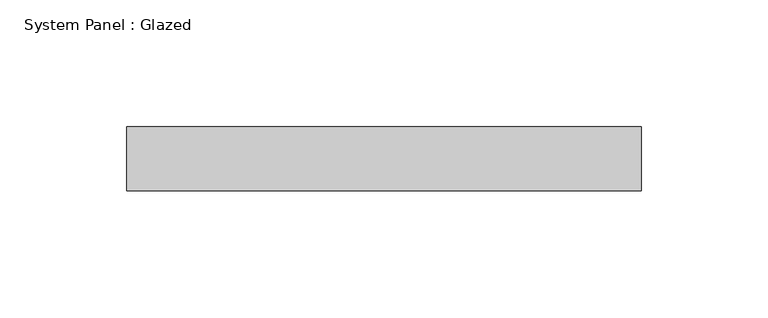
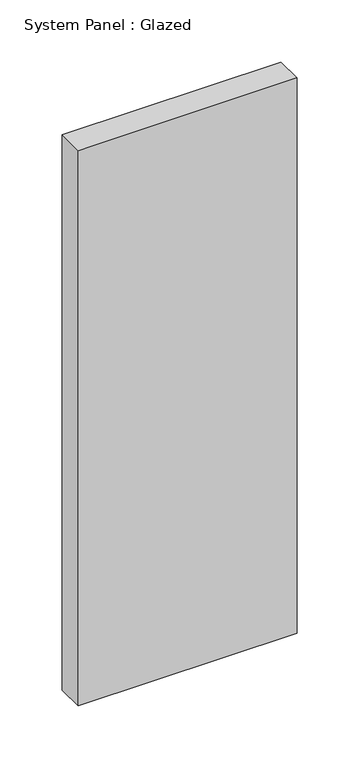
"""IFC4 building model written with IfcOpenShell, lengths in millimetres: plate geometry, System Panel : Glazed."""

from ifc_helpers import new_model, si_unit, origin, origin_with_axes, place, context, project, spatial, polyline, outline, extrude, source, transform, mapped, element, save


def system_panel_glazed_ce347581(model_context):
    return source(origin(), model_context, "Body", "SweptSolid", [
        extrude(outline(polyline([(101.6, 19.05), (-101.6, 19.05), (-101.6, 44.45), (101.6, 44.45), (101.6, 19.05)])), origin_with_axes(), (0.0, 0.0, 1.0), 544.4575706),
    ])


if __name__ == "__main__":
    model = new_model("IFC4")
    model_context = context("Model", 3, world=origin())
    ifc_project = project(units=[si_unit("LENGTHUNIT", "METRE", prefix="MILLI")], contexts=[model_context])
    site = spatial("IfcSite", under=ifc_project)
    building = spatial("IfcBuilding", under=site)
    placement = place(None, origin())
    system_panel_glazed_shape = system_panel_glazed_ce347581(model_context)
    element("IfcPlate", 1, ObjectType="System Panel : Glazed", at=placement, inside=building, context=model_context, shape_type="MappedRepresentation", body=[
        mapped(system_panel_glazed_shape, transform((0.0, 0.0, 0.0), x_axis=(1.0, 0.0, 0.0), y_axis=(0.0, 1.0, 0.0), z_axis=(0.0, 0.0, 1.0))),
    ])
    save(model, "model.ifc")

# Revit data of these elements
# Type "System Panel : Glazed"
#   Construction Type Id = "GSP4R"
#   Analytic Construction = "1/8 in Pilkington single glazing"
#   Visual Light Transmittance = 0.9
#   Solar Heat Gain Coefficient = 0.86
#   Heat Transfer Coefficient (U) = 1.18115 BTU/(h·ft²·°F)
#   Define Thermal Properties by = 1
# Element 1 (IfcPlate, "System Panel : Glazed")
#   Materials on its faces: "Glass"
# Materials
#   "Glass": class "Glass", colour RGB 0 128 192, transparency 0.75, Description = "Soda Lime Glass", Cost = 0
